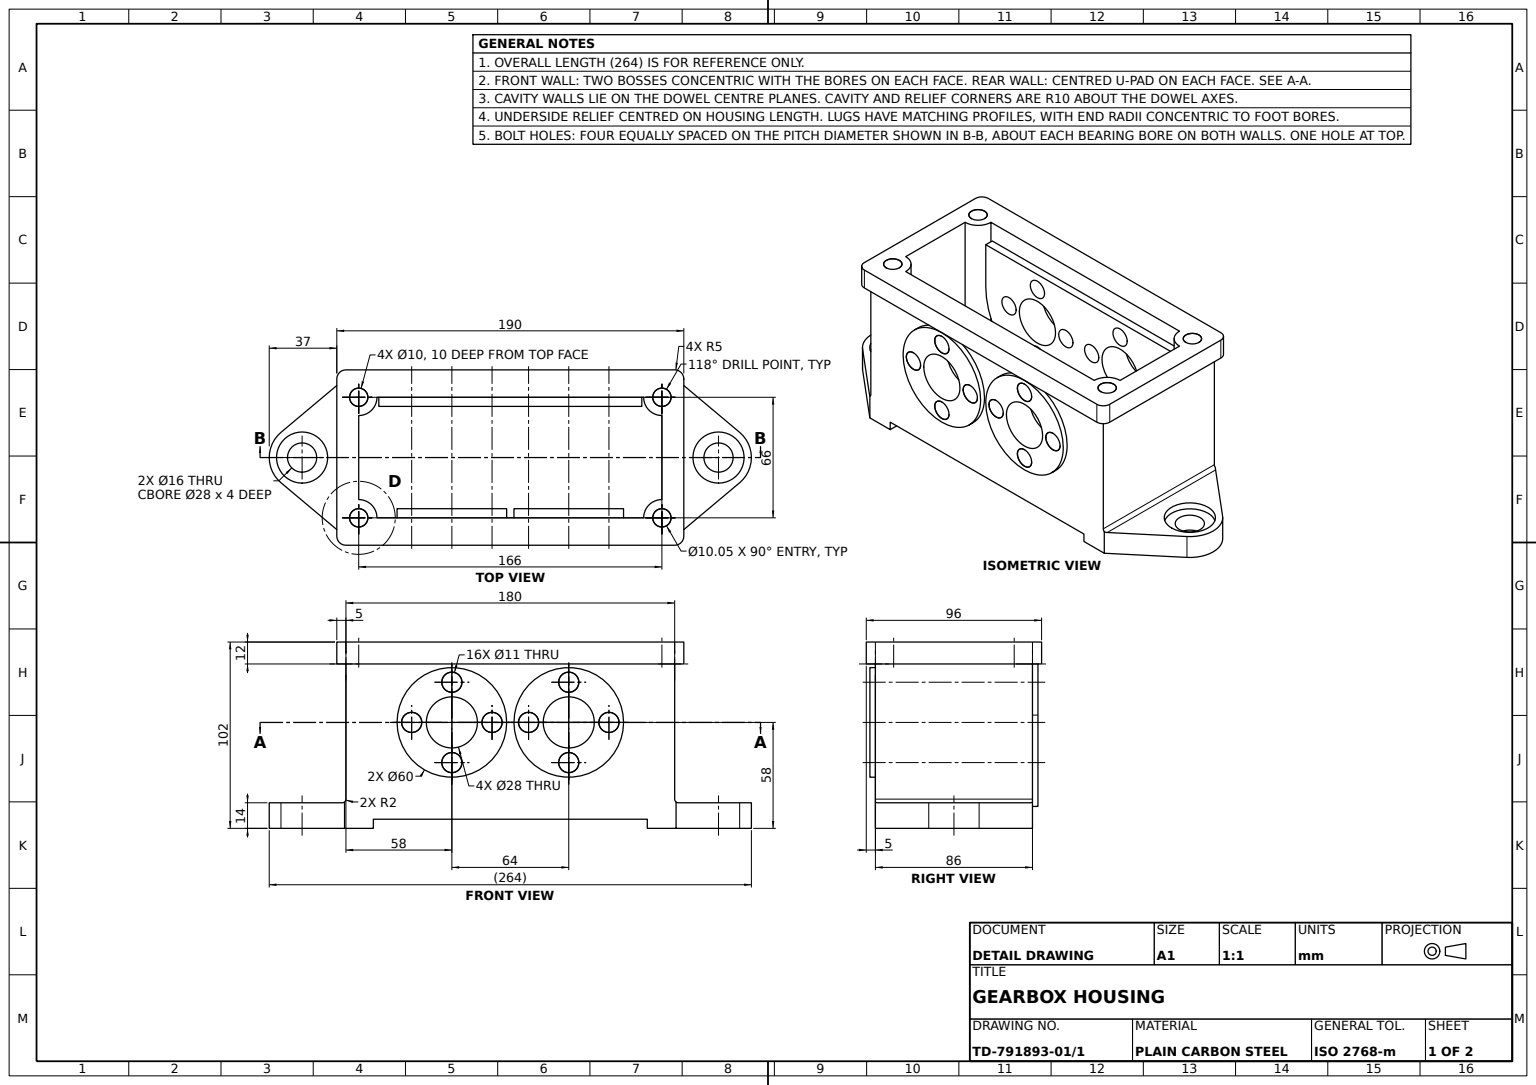
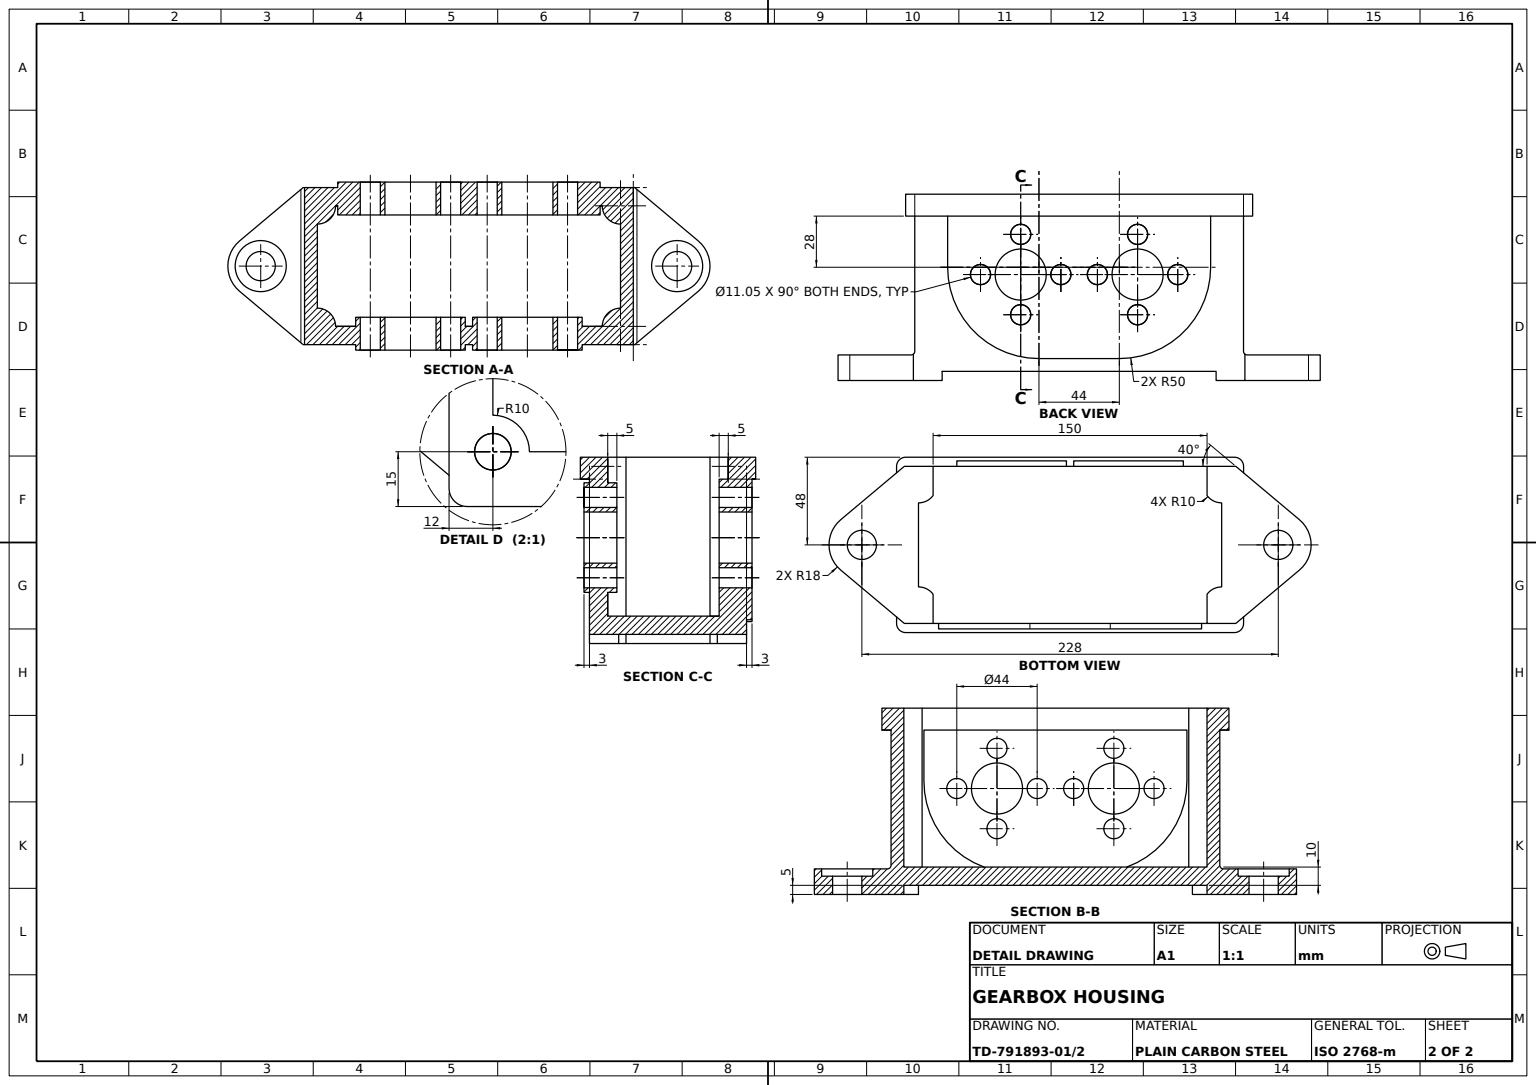
from build123d import *

# Parameters (mm, degrees)
HOUSING_BASE_PROFILE_SKETCH_W          = 180
HOUSING_BASE_PROFILE_SKETCH_H          = 86
HOUSING_BODY_DEPTH                     = 102
TOP_START                              = -12
TOP_FLANGE_DEPTH                       = 12
MOUNTING_FOOT_LUGS_DEPTH               = 14
SIDE_START                             = 3
SIDE_FLANGE_PAD_SKETCH_R               = 14
SIDE_FLANGE_PADS_DEPTH                 = 18
BEARING_START                          = -15
BEARING_BOSS_60_SKETCH_R               = 30
BEARING_BOSS_60_SKETCH_R_2             = 14
BEARING_BOSSES_60_DEPTH                = 18
SKETCH6_2_R                            = 14
BEARING_BORES_DEPTH                    = 191.023682735
HOUSING_CAVITY_SKETCH_W                = 150
HOUSING_CAVITY_SKETCH_H                = 5
HOUSING_CAVITY_DEPTH                   = 191.023682735
BASE_START                             = 5
BASE_PROFILE_PAD_10MM_DEPTH            = 10
FOOT_COUNTERBORED_HOLES_16_D           = 16
FOOT_COUNTERBORED_HOLES_16_CBORE_D     = 28
FOOT_COUNTERBORED_HOLES_16_CBORE_DEPTH = 4
DOWEL_HOLES_10_D                       = 10
DOWEL_HOLES_10_DEPTH                   = 10
DOWEL_HOLES_10_CSINK_D                 = 10.05
DOWEL_HOLES_10_CSINK_ANGLE             = 90
DOWEL_HOLES_10_TIP                     = 3.004303095
FLANGE_BOLT_HOLES_M10_D                = 11
FLANGE_BOLT_HOLES_M10_DEPTH            = 18
FLANGE_BOLT_HOLES_M10_CSINK_D          = 11.05
FLANGE_BOLT_HOLES_M10_CSINK_ANGLE      = 90
FOOT_FILLETS_R2_R                      = 2


with BuildPart() as part:
    # Housing Base Profile Sketch → Housing Body (new body)
    with BuildSketch(Plane(origin=(0, 0, 0), x_dir=(1, 0, 0), z_dir=(0, 1, 0))):
        Rectangle(HOUSING_BASE_PROFILE_SKETCH_W, HOUSING_BASE_PROFILE_SKETCH_H)
        with BuildLine():
            Line((-73, 33), (73, 33))
            ThreePointArc((73, 33), (75.928932188, 25.928932188), (83, 23))
            Line((83, 23), (83, -23))
            ThreePointArc((83, -23), (75.928932188, -25.928932188), (73, -33))
            Line((73, -33), (-73, -33))
            ThreePointArc((-73, -33), (-75.928932188, -25.928932188), (-83, -23))
            Line((-83, -23), (-83, 23))
            ThreePointArc((-83, 23), (-75.928932188, 25.928932188), (-73, 33))
        make_face(mode=Mode.SUBTRACT)
    extrude(amount=HOUSING_BODY_DEPTH)

    # Top Flange Sketch → Top Flange (add)
    with BuildSketch(Plane(origin=(0, 102, 0), x_dir=(1, 0, 0), z_dir=(0, 1, 0)).offset(TOP_START)):
        with BuildLine():
            Line((-90, 48), (90, 48))
            ThreePointArc((90, 48), (93.535533906, 46.535533906), (95, 43))
            Line((95, 43), (95, -43))
            ThreePointArc((95, -43), (93.535533906, -46.535533906), (90, -48))
            Line((90, -48), (-90, -48))
            ThreePointArc((-90, -48), (-93.535533906, -46.535533906), (-95, -43))
            Line((-95, -43), (-95, 43))
            ThreePointArc((-95, 43), (-93.535533906, 46.535533906), (-90, 48))
        make_face()
        with BuildLine():
            Line((-73, 33), (73, 33))
            ThreePointArc((73, 33), (75.928932188, 25.928932188), (83, 23))
            Line((83, 23), (83, -23))
            ThreePointArc((83, -23), (75.928932188, -25.928932188), (73, -33))
            Line((73, -33), (-73, -33))
            ThreePointArc((-73, -33), (-75.928932188, -25.928932188), (-83, -23))
            Line((-83, -23), (-83, 23))
            ThreePointArc((-83, 23), (-75.928932188, 25.928932188), (-73, 33))
        make_face(mode=Mode.SUBTRACT)
    extrude(amount=TOP_FLANGE_DEPTH)

    # Sketch2_4 → Mounting Foot Lugs (add)
    with BuildSketch(Plane(origin=(0, 0, 0), x_dir=(1, 0, 0), z_dir=(0, 1, 0))):
        with BuildLine():
            Line((-90, -43), (-90, 43))
            Line((-90, 43), (-90.757624402, 43))
            Line((-90.757624402, 43), (-125.570176974, 13.788799976))
            ThreePointArc((-125.570176974, 13.788799976), (-132, 0), (-125.570176974, -13.788799976))
            Line((-125.570176974, -13.788799976), (-90.757624402, -43))
            Line((-90.757624402, -43), (-90, -43))
        make_face()
        with BuildLine():
            Line((90.757624402, 43), (90, 43))
            Line((90, 43), (90, -43))
            Line((90, -43), (90.757624402, -43))
            Line((90.757624402, -43), (125.570176974, -13.788799976))
            ThreePointArc((125.570176974, -13.788799976), (132, 0), (125.570176974, 13.788799976))
            Line((125.570176974, 13.788799976), (90.757624402, 43))
        make_face()
    extrude(amount=MOUNTING_FOOT_LUGS_DEPTH)

    # Side Flange Pad Sketch → Side Flange Pads (add)
    # profile 1 of 2: a face of its own
    with BuildSketch(Plane.XY.offset(43).offset(SIDE_START)):
        with BuildLine():
            Line((-22, 12), (0, 12))
            Line((0, 12), (0, 90))
            Line((0, 90), (-72, 90))
            Line((-72, 90), (-72, 62))
            ThreePointArc((-72, 62), (-57.355339059, 26.644660941), (-22, 12))
        make_face()
        with Locations((-32, 58)):
            Circle(SIDE_FLANGE_PAD_SKETCH_R, mode=Mode.SUBTRACT)
    # profile 2 of 2: a face of its own
    with BuildSketch(Plane.XY.offset(43).offset(SIDE_START)):
        with BuildLine():
            Line((0, 90), (0, 12))
            Line((0, 12), (22, 12))
            ThreePointArc((22, 12), (57.355339059, 26.644660941), (72, 62))
            Line((72, 62), (72, 90))
            Line((72, 90), (0, 90))
        make_face()
        with Locations((32, 58)):
            Circle(SIDE_FLANGE_PAD_SKETCH_R, mode=Mode.SUBTRACT)
    extrude(amount=-SIDE_FLANGE_PADS_DEPTH)

    # Bearing Boss _60 Sketch → Bearing Bosses _60 (add)
    # profile 1 of 2: a face of its own
    with BuildSketch(Plane(origin=(0, 0, -43), x_dir=(-1, 0, 0), z_dir=(0, 0, -1)).offset(BEARING_START)):
        with Locations((-32, 58)):
            Circle(BEARING_BOSS_60_SKETCH_R)
        with Locations(Location((-32, 58, 0), (0, 0, 180))):
            Circle(BEARING_BOSS_60_SKETCH_R_2, mode=Mode.SUBTRACT)
    # profile 2 of 2: a face of its own
    with BuildSketch(Plane(origin=(0, 0, -43), x_dir=(-1, 0, 0), z_dir=(0, 0, -1)).offset(BEARING_START)):
        with Locations((32, 58)):
            Circle(BEARING_BOSS_60_SKETCH_R)
        with Locations(Location((32, 58, 0), (0, 0, 180))):
            Circle(BEARING_BOSS_60_SKETCH_R_2, mode=Mode.SUBTRACT)
    extrude(amount=BEARING_BOSSES_60_DEPTH)

    # Sketch6_2 → Bearing Bores (cut, through all)
    with BuildSketch(Plane(origin=(0, 0, -43), x_dir=(-1, 0, 0), z_dir=(0, 0, -1))):
        with Locations(Location((32, 58, 0), (0, 0, 180))):
            Circle(SKETCH6_2_R)
        with Locations(Location((-32, 58, 0), (0, 0, 180))):
            Circle(SKETCH6_2_R)
    extrude(amount=-BEARING_BORES_DEPTH, mode=Mode.SUBTRACT)

    # Housing Cavity Sketch → Housing Cavity (cut, through all)
    with BuildSketch(Plane.XY.offset(43)):
        with Locations((0, 2.5)):
            Rectangle(HOUSING_CAVITY_SKETCH_W, HOUSING_CAVITY_SKETCH_H)
    extrude(amount=-HOUSING_CAVITY_DEPTH, mode=Mode.SUBTRACT)

    # Sketch2_5 → Base Profile Pad 10mm (add)
    with BuildSketch(Plane(origin=(0, 0, 0), x_dir=(1, 0, 0), z_dir=(0, 1, 0)).offset(BASE_START)):
        with BuildLine():
            Line((-83, 23), (-83, -23))
            ThreePointArc((-83, -23), (-75.928932188, -25.928932188), (-73, -33))
            Line((-73, -33), (73, -33))
            ThreePointArc((73, -33), (75.928932188, -25.928932188), (83, -23))
            Line((83, -23), (83, 23))
            ThreePointArc((83, 23), (75.928932188, 25.928932188), (73, 33))
            Line((73, 33), (-73, 33))
            ThreePointArc((-73, 33), (-75.928932188, 25.928932188), (-83, 23))
        make_face()
    extrude(amount=BASE_PROFILE_PAD_10MM_DEPTH)

    # Foot Counterbored Holes _16 (through all)
    with Locations(Plane(origin=(0, 14, 0), x_dir=(1, 0, 0), z_dir=(0, 1, 0))):
        with Locations((114, 0), (-114, 0)):
            CounterBoreHole(FOOT_COUNTERBORED_HOLES_16_D / 2, FOOT_COUNTERBORED_HOLES_16_CBORE_D / 2, FOOT_COUNTERBORED_HOLES_16_CBORE_DEPTH)

    # Dowel Holes _10
    with Locations(Plane(origin=(0, 102, 0), x_dir=(1, 0, 0), z_dir=(0, 1, 0))):
        with Locations((83, 33), (83, -33), (-83, -33), (-83, 33)):
            CounterSinkHole(DOWEL_HOLES_10_D / 2, DOWEL_HOLES_10_CSINK_D / 2, depth=DOWEL_HOLES_10_DEPTH, counter_sink_angle=DOWEL_HOLES_10_CSINK_ANGLE)
            with Locations((0, 0, -(DOWEL_HOLES_10_DEPTH + DOWEL_HOLES_10_TIP / 2))):  # 118° drill point
                Cone(0, DOWEL_HOLES_10_D / 2, DOWEL_HOLES_10_TIP, mode=Mode.SUBTRACT)

    # Flange Bolt Holes M10
    with Locations(Plane.XY.offset(46)):
        with Locations((54, 58), (-32, 80), (-10, 58), (-32, 36), (-54, 58), (32, 36), (10, 58), (32, 80)):
            flange_bolt_holes_m10 = CounterSinkHole(FLANGE_BOLT_HOLES_M10_D / 2, FLANGE_BOLT_HOLES_M10_CSINK_D / 2, depth=FLANGE_BOLT_HOLES_M10_DEPTH, counter_sink_angle=FLANGE_BOLT_HOLES_M10_CSINK_ANGLE)

    # Flange Bolt Holes Mirror: Flange Bolt Holes M10 across plane
    add(flange_bolt_holes_m10.mirror(Plane.XY), mode=Mode.SUBTRACT)

    # Foot Fillets R2
    foot_fillets_r2_edges = [part.edges().sort_by_distance(p)[0] for p in [
        (-90, 14, 0),
        (90, 14, 0),
    ]]
    fillet(foot_fillets_r2_edges, radius=FOOT_FILLETS_R2_R)


solid = part.part
